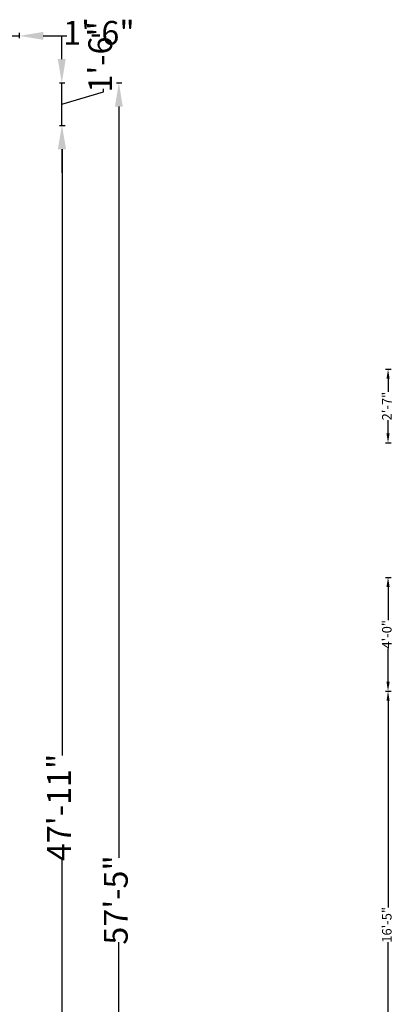
# Model space of a CAD drawing. Units: inches. Extents: x -638 to 186, y -762 to 59.
# Tile 31 of 31: x 29 to 186, y -413 to 3. Entities that reach past the tile are written whole.
import ezdxf

# ---------------------------------------------------------------- set-up
doc = ezdxf.new("R2010")
doc.units = ezdxf.units.IN
doc.layers.add('A-ANNO-DIMS', color=2, linetype='Continuous', lineweight=18)
doc.styles.get("Standard").update_dxf_attribs({"font": 'arial.ttf'})
doc.dimstyles.new('ISO-25', dxfattribs={"dimtxt": 4, "dimasz": 4, "dimexe": 1.25, "dimexo": 0.625, "dimtad": 0, "dimlunit": 4, "dimtxsty": 'Standard', "dimcen": 2.5, "dimclrt": 256, "dimadec": 0, "dimazin": 0, "dimtfac": 1, "dimtmove": 0, "dimatfit": 3, "dimfxl": 1, "dimfxlon": 1, "dimarcsym": 0})

# ---------------------------------------------------------------- blocks, each defined once
blk = doc.blocks.new('*D10')
at = {"layer": 'A-ANNO-DIMS', "color": 0, "lineweight": -2, "transparency": 16777216}
for p, q in [((10.47, -5.21), (10.47, -2.96)), ((28.47, -5.21), (28.47, -2.96)), ((0.47, -4.21), (-9.53, -4.21)), ((10.47, -4.21), (28.47, -4.21)), ((38.47, -4.21), (48.47, -4.21))]:
    blk.add_line(p, q, dxfattribs=at)
at = {"layer": 'A-ANNO-DIMS', "color": 0, "lineweight": 30, "transparency": 16777216}
for points in [[(0.47, -2.54), (0.47, -5.88), (10.47, -4.21)], [(38.47, -2.54), (38.47, -5.88), (28.47, -4.21)]]:
    blk.add_solid(points, dxfattribs=at)
at = {"layer": 'Defpoints', "color": 0, "lineweight": 30, "transparency": 16777216}
for p in [(28.47, -4.21), (10.47, -42.03), (28.47, -42.03)]:
    blk.add_point(p, dxfattribs=at)
at = {"layer": 'A-ANNO-DIMS', "color": 0, "transparency": 16777216, "insert": (61.92, -4.21), "char_height": 10, "attachment_point": 5}
blk.add_mtext('1\'-6"', dxfattribs=at)
blk = doc.blocks.new('*D13')
at = {"layer": 'A-ANNO-DIMS', "color": 0, "lineweight": -2, "transparency": 16777216}
for p, q in [((46.29, -14.03), (46.29, -4.03)), ((45.29, -24.03), (47.54, -24.03)), ((46.29, -42.03), (46.29, -24.03)), ((46.29, -42.03), (46.29, -24.03)), ((46.29, -33.03), (63.79, -27.78)), ((63.79, -27.78), (63.79, -26.53)), ((45.29, -42.03), (47.54, -42.03)), ((46.29, -52.03), (46.29, -62.03))]:
    blk.add_line(p, q, dxfattribs=at)
at = {"layer": 'A-ANNO-DIMS', "color": 0, "lineweight": 30, "transparency": 16777216}
for points in [[(44.62, -14.03), (47.95, -14.03), (46.29, -24.03)], [(44.62, -52.03), (47.95, -52.03), (46.29, -42.03)]]:
    blk.add_solid(points, dxfattribs=at)
at = {"layer": 'Defpoints', "color": 0, "lineweight": 30, "transparency": 16777216}
for p in [(10.47, -24.03), (46.29, -24.03), (10.47, -42.03)]:
    blk.add_point(p, dxfattribs=at)
at = {"layer": 'A-ANNO-DIMS', "color": 0, "transparency": 16777216, "insert": (63.79, -13.09), "char_height": 10, "attachment_point": 5, "rotation": 90}
blk.add_mtext('1\'-6"', dxfattribs=at)
blk = doc.blocks.new('*D14')
at = {"layer": 'A-ANNO-DIMS', "color": 0, "lineweight": -2, "transparency": 16777216}
for p, q in [((45.41, -42.03), (47.66, -42.03)), ((46.41, -52.03), (46.41, -307.65)), ((46.41, -607.03), (46.41, -351.42)), ((45.41, -617.03), (47.66, -617.03))]:
    blk.add_line(p, q, dxfattribs=at)
at = {"layer": 'A-ANNO-DIMS', "color": 0, "lineweight": 30, "transparency": 16777216}
for points in [[(44.74, -52.03), (48.08, -52.03), (46.41, -42.03)], [(44.74, -607.03), (48.08, -607.03), (46.41, -617.03)]]:
    blk.add_solid(points, dxfattribs=at)
at = {"layer": 'Defpoints', "color": 0, "lineweight": 30, "transparency": 16777216}
for p in [(10.47, -42.03), (10.47, -617.03), (46.41, -617.03)]:
    blk.add_point(p, dxfattribs=at)
at = {"layer": 'A-ANNO-DIMS', "color": 0, "transparency": 16777216, "insert": (46.41, -329.53), "char_height": 10, "attachment_point": 5, "rotation": 90}
blk.add_mtext('47\'-11"', dxfattribs=at)
blk = doc.blocks.new('*D15')
at = {"layer": 'A-ANNO-DIMS', "color": 0, "lineweight": -2, "transparency": 16777216}
for p, q in [((69.33, -24.03), (71.58, -24.03)), ((70.33, -34.03), (70.33, -350.73)), ((70.33, -703.03), (70.33, -386.33)), ((69.33, -713.03), (71.58, -713.03))]:
    blk.add_line(p, q, dxfattribs=at)
at = {"layer": 'A-ANNO-DIMS', "color": 0, "lineweight": 30, "transparency": 16777216}
for points in [[(68.66, -34.03), (72, -34.03), (70.33, -24.03)], [(68.66, -703.03), (72, -703.03), (70.33, -713.03)]]:
    blk.add_solid(points, dxfattribs=at)
at = {"layer": 'Defpoints', "color": 0, "lineweight": 30, "transparency": 16777216}
for p in [(-24.67, -24.03), (-10.56, -713.03), (70.33, -713.03)]:
    blk.add_point(p, dxfattribs=at)
at = {"layer": 'A-ANNO-DIMS', "color": 0, "transparency": 16777216, "insert": (70.33, -368.53), "char_height": 10, "attachment_point": 5, "rotation": 90}
blk.add_mtext('57\'-5"', dxfattribs=at)
blk = doc.blocks.new('*D37')
at = {"layer": 'A-ANNO-DIMS', "color": 0, "lineweight": -2, "transparency": 16777216}
for p, q in [((182.66, -232.53), (184.91, -232.53)), ((183.66, -236.53), (183.66, -250.51)), ((183.66, -276.53), (183.66, -262.56)), ((182.66, -280.53), (184.91, -280.53))]:
    blk.add_line(p, q, dxfattribs=at)
at = {"layer": 'A-ANNO-DIMS', "color": 0, "lineweight": 30, "transparency": 16777216}
for points in [[(183, -236.53), (184.33, -236.53), (183.66, -232.53)], [(183, -276.53), (184.33, -276.53), (183.66, -280.53)]]:
    blk.add_solid(points, dxfattribs=at)
at = {"layer": 'Defpoints', "color": 0, "lineweight": 30, "transparency": 16777216}
for p in [(-404.53, -232.53), (-404.53, -280.53), (183.66, -280.53)]:
    blk.add_point(p, dxfattribs=at)
at = {"layer": 'A-ANNO-DIMS', "transparency": 16777216, "insert": (183.66, -256.53), "char_height": 4, "attachment_point": 5, "rotation": 90}
blk.add_mtext('4\'-0"', dxfattribs=at)
blk = doc.blocks.new('*D38')
at = {"layer": 'A-ANNO-DIMS', "color": 0, "lineweight": -2, "transparency": 16777216}
for p, q in [((182.66, -280.53), (184.91, -280.53)), ((183.66, -284.53), (183.66, -371.73)), ((183.66, -473.53), (183.66, -386.34)), ((182.66, -477.53), (184.91, -477.53))]:
    blk.add_line(p, q, dxfattribs=at)
at = {"layer": 'A-ANNO-DIMS', "color": 0, "lineweight": 30, "transparency": 16777216}
for points in [[(183, -284.53), (184.33, -284.53), (183.66, -280.53)], [(183, -473.53), (184.33, -473.53), (183.66, -477.53)]]:
    blk.add_solid(points, dxfattribs=at)
at = {"layer": 'Defpoints', "color": 0, "lineweight": 30, "transparency": 16777216}
for p in [(-404.53, -280.53), (-404.53, -477.53), (183.66, -477.53)]:
    blk.add_point(p, dxfattribs=at)
at = {"layer": 'A-ANNO-DIMS', "transparency": 16777216, "insert": (183.66, -379.03), "char_height": 4, "attachment_point": 5, "rotation": 90}
blk.add_mtext('16\'-5"', dxfattribs=at)
blk = doc.blocks.new('*D49')
at = {"layer": 'A-ANNO-DIMS', "color": 0, "lineweight": -2, "transparency": 16777216}
for p, q in [((182.66, -144.8), (184.91, -144.8)), ((183.66, -148.8), (183.66, -154.33)), ((183.66, -171.81), (183.66, -166.28)), ((182.66, -175.81), (184.91, -175.81))]:
    blk.add_line(p, q, dxfattribs=at)
at = {"layer": 'A-ANNO-DIMS', "color": 0, "lineweight": 30, "transparency": 16777216}
for points in [[(183, -148.8), (184.33, -148.8), (183.66, -144.8)], [(183, -171.81), (184.33, -171.81), (183.66, -175.81)]]:
    blk.add_solid(points, dxfattribs=at)
at = {"layer": 'Defpoints', "color": 0, "lineweight": 30, "transparency": 16777216}
for p in [(-242.35, -144.8), (-242.35, -175.81), (183.66, -175.81)]:
    blk.add_point(p, dxfattribs=at)
at = {"layer": 'A-ANNO-DIMS', "transparency": 16777216, "insert": (183.66, -160.31), "char_height": 4, "attachment_point": 5, "rotation": 90}
blk.add_mtext('2\'-7"', dxfattribs=at)

msp = doc.modelspace()

# ---------------------------------------------------------------- dimensions: what is measured, and where the dimension line sits
at = {"layer": 'A-ANNO-DIMS'}
dim = msp.add_linear_dim(base=(28.474, -4.209), p1=(10.474, -42.033), p2=(28.474, -42.033), dimstyle='ISO-25', override={"dimtxt": 10, "dimasz": 10, "dimclrd": 0, "dimclre": 0, "dimclrt": 0}, dxfattribs=at)
dim.commit()
dim.dimension.update_dxf_attribs({"geometry": '*D10', "text_midpoint": (61.92, -4.209)})
for base, p1, p2, override, picture, middle in [((46.286, -24.033), (10.474, -42.033), (10.474, -24.033), {"dimtxt": 10, "dimasz": 10, "dimclrd": 0, "dimclre": 0, "dimclrt": 0, "dimtmove": 1}, '*D13', (63.791, -25.907)), ((70.331, -713.033), (-24.669, -24.033), (-10.563, -713.033), {"dimtxt": 10, "dimasz": 10, "dimclrd": 0, "dimclre": 0, "dimclrt": 0}, '*D15', (70.331, -368.533)), ((46.411, -617.033), (10.474, -42.033), (10.474, -617.033), {"dimtxt": 10, "dimasz": 10, "dimclrd": 0, "dimclre": 0, "dimclrt": 0}, '*D14', (46.411, -329.533)), ((183.663, -175.813), (-242.352, -144.803), (-242.352, -175.813), {"dimdec": 1, "dimlfac": 1, "dimrnd": 0, "dimzin": 1, "dimdsep": 46, "dimlunit": 4, "dimfrac": 2}, '*D49', (183.663, -160.308)), ((183.663, -280.533), (-404.526, -232.533), (-404.526, -280.533), {"dimdec": 1, "dimlfac": 1, "dimrnd": 0, "dimzin": 1, "dimdsep": 46, "dimlunit": 4, "dimfrac": 2}, '*D37', (183.663, -256.533)), ((183.663, -477.533), (-404.526, -280.533), (-404.526, -477.533), {"dimdec": 1, "dimlfac": 1, "dimrnd": 0, "dimzin": 1, "dimdsep": 46, "dimlunit": 4, "dimfrac": 2}, '*D38', (183.663, -379.033))]:
    dim = msp.add_linear_dim(base=base, p1=p1, p2=p2, angle=90, dimstyle='ISO-25', override=override, dxfattribs=at)
    dim.commit()
    dim.dimension.update_dxf_attribs({"geometry": picture, "text_midpoint": middle})

doc.saveas('drawing.dxf')
